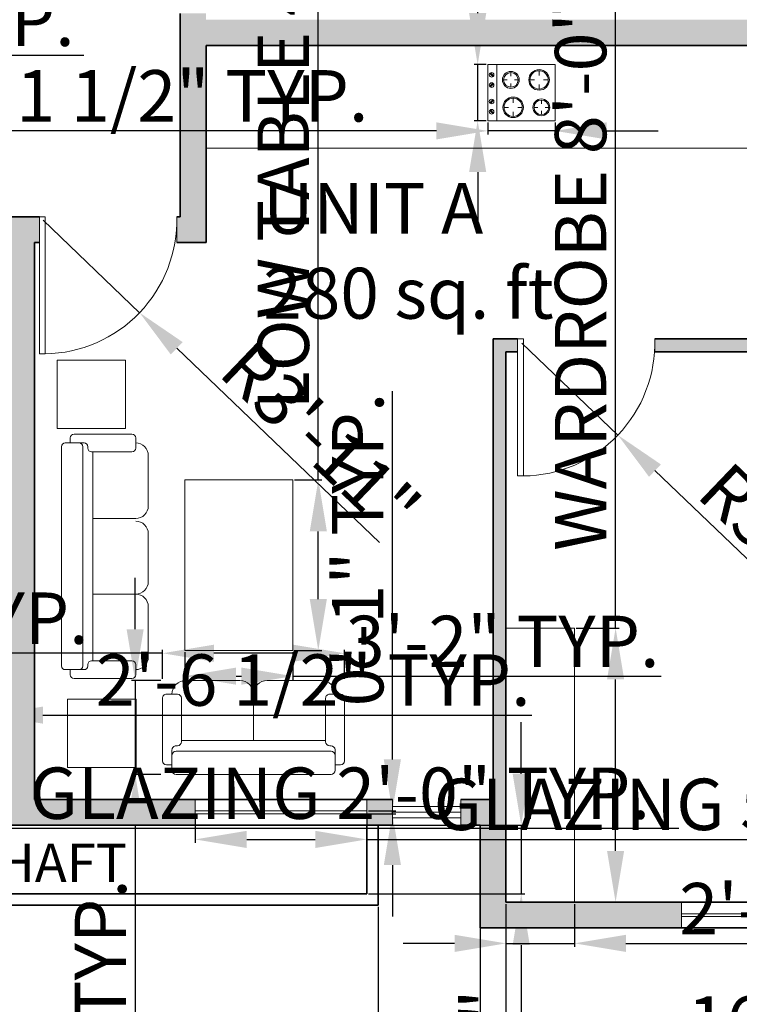
# Model space of a CAD drawing. Units: inches. Extents: x 2043 to 3177, y 1429 to 2563.
# Tile 7 of 14: x 2607 to 2858, y 1608 to 1952. Entities that reach past the tile are written whole.
import ezdxf

# ---------------------------------------------------------------- set-up
doc = ezdxf.new("R2010")
doc.units = ezdxf.units.IN
for name, color, linetype, lineweight in [('A-ANNO-DIMS', 2, 'Continuous', 13), ('A-AREA-IDEN', 7, 'Continuous', 18), ('A-DOOR', 3, 'Continuous', 18), ('A-EQPM', 8, 'Continuous', 18), ('A-FLOR-CASE', 8, 'Continuous', 18), ('A-FURN', 8, 'Continuous', 18), ('A-GLAZ', 4, 'Continuous', 18), ('A-WALL', 7, 'Continuous', 35)]:
    doc.layers.add(name, color=color, linetype=linetype, lineweight=lineweight)
doc.layers.add('A-WALL-PATT', color=251, linetype='Continuous', lineweight=13, true_color=0x636466)
doc.styles.get("Standard").update_dxf_attribs({"font": 'arial.ttf'})
doc.dimstyles.new('ISO-25', dxfattribs={"dimtxt": 18, "dimasz": 18, "dimexe": 1.25, "dimexo": 0.625, "dimtad": 1, "dimlunit": 3, "dimtxsty": 'Standard', "dimcen": 2.5, "dimadec": 0, "dimazin": 0, "dimtfac": 1, "dimtmove": 0, "dimatfit": 3, "dimfxl": 1, "dimarcsym": 0})

# ---------------------------------------------------------------- blocks, each defined once
blk = doc.blocks.new('A$C115861F8')
for p, q in [((0.0679, 0.6401), (0.0679, 0.6013)), ((1.7846, 0.6692), (0.097, 0.6692)), ((1.8136, 0.6401), (1.8136, 0.6013)), ((0, 0.5722), (0, 0.1261)), ((0.0679, 0.6013), (0.0291, 0.6013)), ((0.0679, 0.5334), (0.0679, 0.6013)), ((0.0679, 0.4946), (0.0679, 0.5431)), ((1.8136, 0.6013), (1.8524, 0.6013)), ((1.8136, 0.5334), (1.8136, 0.6013)), ((1.8136, 0.4946), (1.8136, 0.5431)), ((1.8815, 0.5722), (1.8815, 0.1261)), ((1.7846, 0.5043), (0.097, 0.5043)), ((0.1067, 0.4655), (0.097, 0.4655)), ((1.7749, 0.4655), (1.7846, 0.4655)), ((0.1358, 0.1261), (0.1358, 0.4364)), ((1.7458, 0.4267), (0.1358, 0.4267)), ((0.6498, 0.097), (0.6498, 0.4267)), ((1.2317, 0.097), (1.2317, 0.4267)), ((1.7458, 0.1261), (1.7458, 0.4364)), ((0.0291, 0.097), (0.1067, 0.097)), ((1.8524, 0.097), (1.7749, 0.097)), ((0.1649, 0), (0.5528, 0)), ((1.1347, 0), (0.7468, 0)), ((1.3287, 0), (1.7167, 0))]:
    blk.add_line(p, q)
for centre, radius, start, end in [((0.097, 0.6401), 0.0291, 90, 180), ((1.7846, 0.6401), 0.0291, 0, 90), ((0.0291, 0.5722), 0.0291, 90, 180), ((0.097, 0.5334), 0.0291, 180, 270), ((1.7846, 0.5334), 0.0291, 270, 0), ((1.8524, 0.5722), 0.0291, 0, 90), ((0.097, 0.4946), 0.0291, 180, 270), ((0.1067, 0.4364), 0.0291, 0, 90), ((1.7749, 0.4364), 0.0291, 90, 180), ((1.7846, 0.4946), 0.0291, 270, 0), ((0.0291, 0.1261), 0.0291, 180, 270), ((0.1649, 0.097), 0.097, 180, 270), ((0.1067, 0.1261), 0.0291, 270, 0), ((0.5528, 0.097), 0.097, 270, 0), ((0.7468, 0.097), 0.097, 180, 270), ((1.1147, 0.097), 0.097, 270, 0), ((1.3287, 0.097), 0.097, 180, 270), ((1.7167, 0.097), 0.097, 270, 0), ((1.7749, 0.1261), 0.0291, 180, 270), ((1.8524, 0.1261), 0.0291, 270, 0)]:
    blk.add_arc(centre, radius, start, end)
blk = doc.blocks.new('A$C02A636C4')
for p, q in [((0.0679, 0.6401), (0.0679, 0.6013)), ((1.2026, 0.6692), (0.097, 0.6692)), ((1.2317, 0.6401), (1.2317, 0.6013)), ((0, 0.5722), (0, 0.1261)), ((0.0679, 0.6013), (0.0291, 0.6013)), ((0.0679, 0.5334), (0.0679, 0.6013)), ((1.2317, 0.6013), (1.2705, 0.6013)), ((1.2317, 0.5334), (1.2317, 0.6013)), ((1.2996, 0.5722), (1.2996, 0.1261)), ((0.0679, 0.4946), (0.0679, 0.5431)), ((1.2026, 0.5043), (0.097, 0.5043)), ((1.2317, 0.4946), (1.2317, 0.5431)), ((0.1067, 0.4655), (0.097, 0.4655)), ((0.1358, 0.1261), (0.1358, 0.4364)), ((1.1638, 0.4267), (0.1358, 0.4267)), ((0.6498, 0.097), (0.6498, 0.4267)), ((1.1638, 0.1261), (1.1638, 0.4364)), ((1.1929, 0.4655), (1.2026, 0.4655)), ((0.0291, 0.097), (0.1067, 0.097)), ((1.2705, 0.097), (1.1929, 0.097)), ((0.1649, 0), (0.5528, 0)), ((0.7468, 0), (1.1347, 0))]:
    blk.add_line(p, q)
for centre, radius, start, end in [((0.097, 0.6401), 0.0291, 90, 180), ((1.2026, 0.6401), 0.0291, 0, 90), ((0.0291, 0.5722), 0.0291, 90, 180), ((1.2705, 0.5722), 0.0291, 0, 90), ((0.097, 0.5334), 0.0291, 180, 270), ((0.097, 0.4946), 0.0291, 180, 270), ((1.2026, 0.5334), 0.0291, 270, 0), ((1.2026, 0.4946), 0.0291, 270, 0), ((0.1067, 0.4364), 0.0291, 0, 90), ((1.1929, 0.4364), 0.0291, 90, 180), ((0.0291, 0.1261), 0.0291, 180, 270), ((0.1649, 0.097), 0.097, 180, 270), ((0.1067, 0.1261), 0.0291, 270, 0), ((0.5528, 0.097), 0.097, 270, 0), ((0.7468, 0.097), 0.097, 180, 270), ((1.1347, 0.097), 0.097, 270, 0), ((1.1929, 0.1261), 0.0291, 180, 270), ((1.2705, 0.1261), 0.0291, 270, 0)]:
    blk.add_arc(centre, radius, start, end)
blk = doc.blocks.new('*D20')
at = {"layer": 'A-ANNO-DIMS', "color": 0, "lineweight": -2, "transparency": 16777216}
for p, q in [((2767.74, 1633.77), (2767.74, 1562.86)), ((2980.74, 1633.77), (2980.74, 1562.86)), ((2785.74, 1564.11), (2962.74, 1564.11))]:
    blk.add_line(p, q, dxfattribs=at)
at = {"layer": 'A-ANNO-DIMS', "color": 0, "transparency": 16777216}
for points in [[(2785.74, 1567.11), (2785.74, 1561.11), (2767.74, 1564.11)], [(2962.74, 1567.11), (2962.74, 1561.11), (2980.74, 1564.11)]]:
    blk.add_solid(points, dxfattribs=at)
at = {"layer": 'Defpoints', "color": 0, "transparency": 16777216}
for p in [(2767.74, 1634.39), (2980.74, 1634.39), (2980.74, 1564.11)]:
    blk.add_point(p, dxfattribs=at)
at = {"layer": 'A-ANNO-DIMS', "color": 0, "transparency": 16777216, "insert": (2874.24, 1573.93), "char_height": 18, "attachment_point": 5}
blk.add_mtext('22\'-0"', dxfattribs=at)
blk = doc.blocks.new('*D21')
at = {"layer": 'A-ANNO-DIMS', "color": 0, "lineweight": -2, "transparency": 16777216}
for p, q in [((2731.99, 1641.77), (2731.99, 1511.06)), ((2767.74, 1641.77), (2767.74, 1511.06)), ((2713.99, 1512.31), (2695.99, 1512.31)), ((2731.99, 1512.31), (2767.74, 1512.31)), ((2785.74, 1512.31), (2852.83, 1512.31))]:
    blk.add_line(p, q, dxfattribs=at)
at = {"layer": 'A-ANNO-DIMS', "color": 0, "transparency": 16777216}
for points in [[(2713.99, 1515.31), (2713.99, 1509.31), (2731.99, 1512.31)], [(2785.74, 1515.31), (2785.74, 1509.31), (2767.74, 1512.31)]]:
    blk.add_solid(points, dxfattribs=at)
at = {"layer": 'Defpoints', "color": 0, "transparency": 16777216}
for p in [(2731.99, 1642.39), (2767.74, 1642.39), (2767.74, 1512.31)]:
    blk.add_point(p, dxfattribs=at)
at = {"layer": 'A-ANNO-DIMS', "color": 0, "transparency": 16777216, "insert": (2828.29, 1522.13), "char_height": 18, "attachment_point": 5}
blk.add_mtext('3\'-0"', dxfattribs=at)
blk = doc.blocks.new('*D22')
at = {"layer": 'A-ANNO-DIMS', "color": 0, "lineweight": -2, "transparency": 16777216}
for p, q in [((2482.49, 1641.77), (2482.49, 1560.37)), ((2731.99, 1641.77), (2731.99, 1560.37)), ((2500.49, 1561.62), (2713.99, 1561.62))]:
    blk.add_line(p, q, dxfattribs=at)
at = {"layer": 'A-ANNO-DIMS', "color": 0, "transparency": 16777216}
for points in [[(2500.49, 1564.62), (2500.49, 1558.62), (2482.49, 1561.62)], [(2713.99, 1564.62), (2713.99, 1558.62), (2731.99, 1561.62)]]:
    blk.add_solid(points, dxfattribs=at)
at = {"layer": 'Defpoints', "color": 0, "transparency": 16777216}
for p in [(2482.49, 1642.39), (2731.99, 1642.39), (2731.99, 1561.62)]:
    blk.add_point(p, dxfattribs=at)
at = {"layer": 'A-ANNO-DIMS', "color": 0, "transparency": 16777216, "insert": (2607.24, 1571.44), "char_height": 18, "attachment_point": 5}
blk.add_mtext('25\'-0"', dxfattribs=at)
blk = doc.blocks.new('*D29')
at = {"layer": 'A-ANNO-DIMS', "color": 0, "lineweight": -2, "transparency": 16777216}
for p, q in [((2233.74, 1633.77), (2233.74, 1430.58)), ((2980.74, 1633.77), (2980.74, 1430.58)), ((2251.74, 1431.83), (2962.74, 1431.83))]:
    blk.add_line(p, q, dxfattribs=at)
at = {"layer": 'A-ANNO-DIMS', "color": 0, "transparency": 16777216}
for points in [[(2251.74, 1434.83), (2251.74, 1428.83), (2233.74, 1431.83)], [(2962.74, 1434.83), (2962.74, 1428.83), (2980.74, 1431.83)]]:
    blk.add_solid(points, dxfattribs=at)
at = {"layer": 'Defpoints', "color": 0, "transparency": 16777216}
for p in [(2233.74, 1634.39), (2980.74, 1634.39), (2980.74, 1431.83)]:
    blk.add_point(p, dxfattribs=at)
at = {"layer": 'A-ANNO-DIMS', "color": 0, "transparency": 16777216, "insert": (2607.24, 1441.64), "char_height": 18, "attachment_point": 5}
blk.add_mtext('75\'-0"', dxfattribs=at)
blk = doc.blocks.new('A$C16A60262')
at = {"linetype": 'ByBlock'}
for p, q in [((0, 600), (0, 0)), ((487.7, 600), (0, 600)), ((0, 600), (500, 600)), ((0, 600), (500, 600)), ((500, 600), (500, 0)), ((500, 600), (500, 0)), ((500, 520.4), (0, 520.4)), ((119.4, 455.6), (119.4, 414.9)), ((363.3, 459.6), (363.3, 427.1)), ((38.1, 374.3), (78.8, 374.3)), ((200.7, 374.3), (160.1, 374.3)), ((298.2, 394.6), (330.7, 394.6)), ((363.3, 329.6), (363.3, 362.1)), ((428.3, 394.6), (395.8, 394.6)), ((119.4, 293), (119.4, 333.7)), ((119.4, 188.6), (119.4, 156.1)), ((363.3, 225.2), (363.3, 184.6)), ((54.4, 123.6), (86.9, 123.6)), ((119.4, 58.6), (119.4, 91.1)), ((184.4, 123.6), (151.9, 123.6)), ((282, 143.9), (322.6, 143.9)), ((363.3, 62.6), (363.3, 103.3)), ((444.5, 143.9), (403.9, 143.9)), ((0, 0), (500, 0))]:
    blk.add_line(p, q, dxfattribs=at)
for p, q in [((66.2, 557.5), (87.4, 578.7)), ((71.9, 551.8), (66.2, 557.5)), ((93.1, 573), (71.9, 551.8)), ((87.4, 578.7), (93.1, 573)), ((157.6, 572.5), (163.3, 578.1)), ((178.8, 551.2), (157.6, 572.5)), ((163.3, 578.1), (184.5, 556.9)), ((184.5, 556.9), (178.8, 551.2)), ((305.1, 572.5), (310.8, 578.1)), ((326.3, 551.2), (305.1, 572.5)), ((310.8, 578.1), (332, 556.9)), ((332, 556.9), (326.3, 551.2)), ((396.2, 558.5), (417.4, 579.7)), ((401.9, 552.8), (396.2, 558.5)), ((423.1, 574), (401.9, 552.8)), ((417.4, 579.7), (423.1, 574))]:
    blk.add_line(p, q)
for centre in [(80.1, 565.7), (171.2, 565.7), (317.6, 565.7), (408.7, 565.7)]:
    blk.add_circle(centre, 20.6)
for centre, radius in [((119.4, 374.3), 91.3), ((119.4, 374.3), 81.3), ((363.3, 394.6), 75), ((363.3, 394.6), 65), ((119.4, 123.6), 75), ((119.4, 123.6), 65), ((363.3, 143.9), 91.3), ((363.3, 143.9), 81.3)]:
    blk.add_circle(centre, radius, dxfattribs=at)
blk = doc.blocks.new('WARDROBE-96X24')
for p, q in [((0, 96), (24, 96)), ((24, 96), (24, 0))]:
    blk.add_line(p, q)
blk = doc.blocks.new('END-TABLE-24')
blk.add_lwpolyline([(24, 24), (24, 0), (0, 0), (0, 24)], close=True)
blk = doc.blocks.new('COFFEE-TABLE-RECT')
blk.add_lwpolyline([(0, 59.71), (37.81, 59.71), (37.81, 0), (0, 0)], close=True)
blk = doc.blocks.new('GLAZING-72')
for p, q in [((72, 1), (0, 1)), ((72, 0), (0, 0))]:
    blk.add_line(p, q)
blk = doc.blocks.new('GLAZING-24-TRIPLE')
for p, q in [((24, 4), (0, 4)), ((24, 2), (0, 2)), ((24, 0), (0, 0))]:
    blk.add_line(p, q)
blk = doc.blocks.new('GLAZING-60')
for p, q in [((0, 1), (60, 1)), ((0, 0), (60, 0))]:
    blk.add_line(p, q)
blk = doc.blocks.new('*D41')
at = {"layer": 'A-ANNO-DIMS', "color": 0, "lineweight": -2, "transparency": 16777216}
for p, q in [((2711.06, 1791.23), (2711.06, 2126.25)), ((2702.73, 1791.23), (2712.31, 1791.23)), ((2711.06, 1749.52), (2711.06, 1773.23)), ((2702.73, 1731.52), (2712.31, 1731.52))]:
    blk.add_line(p, q, dxfattribs=at)
at = {"layer": 'A-ANNO-DIMS', "color": 0, "transparency": 16777216}
for points in [[(2708.06, 1773.23), (2714.06, 1773.23), (2711.06, 1791.23)], [(2708.06, 1749.52), (2714.06, 1749.52), (2711.06, 1731.52)]]:
    blk.add_solid(points, dxfattribs=at)
at = {"layer": 'Defpoints', "color": 0, "transparency": 16777216}
for p in [(2702.11, 1791.23), (2711.06, 1791.23), (2702.11, 1731.52)]:
    blk.add_point(p, dxfattribs=at)
at = {"layer": 'A-ANNO-DIMS', "color": 0, "transparency": 16777216, "insert": (2701.13, 1967.74), "char_height": 18, "attachment_point": 5, "rotation": 90}
blk.add_mtext('LOW TABLE 4\'-11 1/2" TYP.', dxfattribs=at)
blk = doc.blocks.new('*D42')
at = {"layer": 'A-ANNO-DIMS', "color": 0, "lineweight": -2, "transparency": 16777216}
for p, q in [((2664.29, 1730.9), (2664.29, 1721.31)), ((2702.11, 1730.9), (2702.11, 1721.31)), ((2682.29, 1722.56), (2684.11, 1722.56)), ((2702.11, 1722.56), (2831.06, 1722.56))]:
    blk.add_line(p, q, dxfattribs=at)
at = {"layer": 'A-ANNO-DIMS', "color": 0, "transparency": 16777216}
for points in [[(2682.29, 1725.56), (2682.29, 1719.56), (2664.29, 1722.56)], [(2684.11, 1725.56), (2684.11, 1719.56), (2702.11, 1722.56)]]:
    blk.add_solid(points, dxfattribs=at)
at = {"layer": 'Defpoints', "color": 0, "transparency": 16777216}
for p in [(2664.29, 1731.52), (2702.11, 1731.52), (2702.11, 1722.56)]:
    blk.add_point(p, dxfattribs=at)
at = {"layer": 'A-ANNO-DIMS', "color": 0, "transparency": 16777216, "insert": (2775.59, 1732.38), "char_height": 18, "attachment_point": 5}
blk.add_mtext('3\'-2" TYP.', dxfattribs=at)
blk = doc.blocks.new('*D44')
at = {"layer": 'A-ANNO-DIMS', "color": 0, "lineweight": -2, "transparency": 16777216}
for p, q in [((2566.23, 1721.12), (2566.23, 1707.66)), ((2596.65, 1721.12), (2596.65, 1707.66)), ((2548.23, 1708.91), (2530.23, 1708.91)), ((2566.23, 1708.91), (2596.65, 1708.91)), ((2614.65, 1708.91), (2785.87, 1708.91))]:
    blk.add_line(p, q, dxfattribs=at)
at = {"layer": 'A-ANNO-DIMS', "color": 0, "transparency": 16777216}
for points in [[(2548.23, 1711.91), (2548.23, 1705.91), (2566.23, 1708.91)], [(2614.65, 1711.91), (2614.65, 1705.91), (2596.65, 1708.91)]]:
    blk.add_solid(points, dxfattribs=at)
at = {"layer": 'Defpoints', "color": 0, "transparency": 16777216}
for p in [(2566.23, 1721.74), (2596.65, 1721.74), (2596.65, 1708.91)]:
    blk.add_point(p, dxfattribs=at)
at = {"layer": 'A-ANNO-DIMS', "color": 0, "transparency": 16777216, "insert": (2709.26, 1718.85), "char_height": 18, "attachment_point": 5}
blk.add_mtext('2\'-6 1/2" TYP.', dxfattribs=at)
blk = doc.blocks.new('*D45')
at = {"layer": 'A-ANNO-DIMS', "color": 0, "lineweight": -2, "transparency": 16777216}
for p, q in [((2656.49, 1721.63), (2656.49, 1731.82)), ((2720.27, 1721.63), (2720.27, 1731.82)), ((2656.49, 1730.57), (2388.57, 1730.57)), ((2702.27, 1730.57), (2674.49, 1730.57))]:
    blk.add_line(p, q, dxfattribs=at)
at = {"layer": 'A-ANNO-DIMS', "color": 0, "transparency": 16777216}
for points in [[(2674.49, 1733.57), (2674.49, 1727.57), (2656.49, 1730.57)], [(2702.27, 1733.57), (2702.27, 1727.57), (2720.27, 1730.57)]]:
    blk.add_solid(points, dxfattribs=at)
at = {"layer": 'Defpoints', "color": 0, "transparency": 16777216}
for p in [(2656.49, 1730.57), (2656.49, 1721), (2720.27, 1721)]:
    blk.add_point(p, dxfattribs=at)
at = {"layer": 'A-ANNO-DIMS', "color": 0, "transparency": 16777216, "insert": (2513.53, 1740.51), "char_height": 18, "attachment_point": 5}
blk.add_mtext('LOVESEAT 5\'-4" TYP.', dxfattribs=at)
blk = doc.blocks.new('*D46')
at = {"layer": 'A-ANNO-DIMS', "color": 0, "lineweight": -2, "transparency": 16777216}
for p, q in [((2646.93, 1739), (2646.93, 1757)), ((2655.87, 1721), (2645.68, 1721)), ((2646.93, 1721), (2646.93, 1688.16)), ((2655.87, 1688.16), (2645.68, 1688.16)), ((2646.93, 1670.16), (2646.93, 1540.89))]:
    blk.add_line(p, q, dxfattribs=at)
at = {"layer": 'A-ANNO-DIMS', "color": 0, "transparency": 16777216}
for points in [[(2643.93, 1739), (2649.93, 1739), (2646.93, 1721)], [(2643.93, 1670.16), (2649.93, 1670.16), (2646.93, 1688.16)]]:
    blk.add_solid(points, dxfattribs=at)
at = {"layer": 'Defpoints', "color": 0, "transparency": 16777216}
for p in [(2656.49, 1721), (2646.93, 1688.16), (2656.49, 1688.16)]:
    blk.add_point(p, dxfattribs=at)
at = {"layer": 'A-ANNO-DIMS', "color": 0, "transparency": 16777216, "insert": (2637.11, 1596.52), "char_height": 18, "attachment_point": 5, "rotation": 90}
blk.add_mtext('2\'-9" TYP.', dxfattribs=at)
blk = doc.blocks.new('*D57')
at = {"layer": 'A-ANNO-DIMS', "color": 0, "lineweight": -2, "transparency": 16777216}
for p, q in [((2309.03, 1935.24), (2309.03, 1941.18)), ((2344.46, 1935.24), (2344.46, 1941.18)), ((2291.03, 1939.93), (2273.03, 1939.93)), ((2309.03, 1939.93), (2344.46, 1939.93)), ((2362.46, 1939.93), (2629.01, 1939.93))]:
    blk.add_line(p, q, dxfattribs=at)
at = {"layer": 'A-ANNO-DIMS', "color": 0, "transparency": 16777216}
for points in [[(2291.03, 1942.93), (2291.03, 1936.93), (2309.03, 1939.93)], [(2362.46, 1942.93), (2362.46, 1936.93), (2344.46, 1939.93)]]:
    blk.add_solid(points, dxfattribs=at)
at = {"layer": 'Defpoints', "color": 0, "transparency": 16777216}
for p in [(2344.46, 1939.93), (2309.03, 1934.62), (2344.46, 1934.62)]:
    blk.add_point(p, dxfattribs=at)
at = {"layer": 'A-ANNO-DIMS', "color": 0, "transparency": 16777216, "insert": (2504.74, 1949.86), "char_height": 18, "attachment_point": 5}
blk.add_mtext('BASIN 2\'-11 1/2" TYP.', dxfattribs=at)
blk = doc.blocks.new('*D61')
at = {"layer": 'A-ANNO-DIMS', "color": 0, "lineweight": -2, "transparency": 16777216}
for p, q in [((2752.39, 1913.46), (2434.98, 1913.46)), ((2770.39, 1916.38), (2770.39, 1912.21)), ((2794.01, 1913.46), (2770.39, 1913.46)), ((2794.01, 1916.38), (2794.01, 1912.21)), ((2812.01, 1913.46), (2830.01, 1913.46))]:
    blk.add_line(p, q, dxfattribs=at)
at = {"layer": 'A-ANNO-DIMS', "color": 0, "transparency": 16777216}
for points in [[(2752.39, 1916.46), (2752.39, 1910.46), (2770.39, 1913.46)], [(2812.01, 1916.46), (2812.01, 1910.46), (2794.01, 1913.46)]]:
    blk.add_solid(points, dxfattribs=at)
at = {"layer": 'Defpoints', "color": 0, "transparency": 16777216}
for p in [(2770.39, 1917.01), (2794.01, 1917.01), (2770.39, 1913.46)]:
    blk.add_point(p, dxfattribs=at)
at = {"layer": 'A-ANNO-DIMS', "color": 0, "transparency": 16777216, "insert": (2584.68, 1923.4), "char_height": 18, "attachment_point": 5}
blk.add_mtext('COOKTOP 1\'-11 1/2" TYP.', dxfattribs=at)
blk = doc.blocks.new('*D62')
at = {"layer": 'A-ANNO-DIMS', "color": 0, "lineweight": -2, "transparency": 16777216}
for p, q in [((2766.85, 1954.69), (2766.85, 2123.91)), ((2769.77, 1936.69), (2765.6, 1936.69)), ((2766.85, 1917.01), (2766.85, 1936.69)), ((2769.77, 1917.01), (2765.6, 1917.01)), ((2766.85, 1899.01), (2766.85, 1881.01))]:
    blk.add_line(p, q, dxfattribs=at)
at = {"layer": 'A-ANNO-DIMS', "color": 0, "transparency": 16777216}
for points in [[(2763.85, 1954.69), (2769.85, 1954.69), (2766.85, 1936.69)], [(2763.85, 1899.01), (2769.85, 1899.01), (2766.85, 1917.01)]]:
    blk.add_solid(points, dxfattribs=at)
at = {"layer": 'Defpoints', "color": 0, "transparency": 16777216}
for p in [(2766.85, 1936.69), (2770.39, 1936.69), (2770.39, 1917.01)]:
    blk.add_point(p, dxfattribs=at)
at = {"layer": 'A-ANNO-DIMS', "color": 0, "transparency": 16777216, "insert": (2756.92, 2048.3), "char_height": 18, "attachment_point": 5, "rotation": 90}
blk.add_mtext('1\'-7 1/2" TYP.', dxfattribs=at)
blk = doc.blocks.new('*D65')
at = {"layer": 'A-ANNO-DIMS', "color": 0, "lineweight": -2, "transparency": 16777216}
for p, q in [((2815.14, 1739.39), (2815.14, 2024.17)), ((2801.37, 1739.39), (2816.39, 1739.39)), ((2815.14, 1661.39), (2815.14, 1721.39)), ((2801.37, 1643.39), (2816.39, 1643.39))]:
    blk.add_line(p, q, dxfattribs=at)
at = {"layer": 'A-ANNO-DIMS', "color": 0, "transparency": 16777216}
for points in [[(2812.14, 1721.39), (2818.14, 1721.39), (2815.14, 1739.39)], [(2812.14, 1661.39), (2818.14, 1661.39), (2815.14, 1643.39)]]:
    blk.add_solid(points, dxfattribs=at)
at = {"layer": 'Defpoints', "color": 0, "transparency": 16777216}
for p in [(2800.74, 1739.39), (2815.14, 1739.39), (2800.74, 1643.39)]:
    blk.add_point(p, dxfattribs=at)
at = {"layer": 'A-ANNO-DIMS', "color": 0, "transparency": 16777216, "insert": (2805.21, 1890.78), "char_height": 18, "attachment_point": 5, "rotation": 90}
blk.add_mtext('WARDROBE 8\'-0" TYP.', dxfattribs=at)
blk = doc.blocks.new('*D66')
at = {"layer": 'A-ANNO-DIMS', "color": 0, "lineweight": -2, "transparency": 16777216}
for p, q in [((2776.74, 1642.77), (2776.74, 1627.74)), ((2800.74, 1642.77), (2800.74, 1627.74)), ((2758.74, 1628.99), (2740.74, 1628.99)), ((2776.74, 1628.99), (2800.74, 1628.99)), ((2818.74, 1628.99), (2948.02, 1628.99))]:
    blk.add_line(p, q, dxfattribs=at)
at = {"layer": 'A-ANNO-DIMS', "color": 0, "transparency": 16777216}
for points in [[(2758.74, 1631.99), (2758.74, 1625.99), (2776.74, 1628.99)], [(2818.74, 1631.99), (2818.74, 1625.99), (2800.74, 1628.99)]]:
    blk.add_solid(points, dxfattribs=at)
at = {"layer": 'Defpoints', "color": 0, "transparency": 16777216}
for p in [(2776.74, 1643.39), (2800.74, 1643.39), (2800.74, 1628.99)]:
    blk.add_point(p, dxfattribs=at)
at = {"layer": 'A-ANNO-DIMS', "color": 0, "transparency": 16777216, "insert": (2892.38, 1638.81), "char_height": 18, "attachment_point": 5}
blk.add_mtext('2\'-0" TYP.', dxfattribs=at)
blk = doc.blocks.new('*D67')
at = {"layer": 'A-ANNO-DIMS', "color": 0, "lineweight": -2, "transparency": 16777216}
for p, q in [((2453.49, 1672.27), (2453.49, 1668.04)), ((2477.49, 1672.27), (2477.49, 1668.04)), ((2435.49, 1669.29), (2417.49, 1669.29)), ((2453.49, 1669.29), (2477.49, 1669.29)), ((2495.49, 1669.29), (2837.31, 1669.29))]:
    blk.add_line(p, q, dxfattribs=at)
at = {"layer": 'A-ANNO-DIMS', "color": 0, "transparency": 16777216}
for points in [[(2435.49, 1672.29), (2435.49, 1666.29), (2453.49, 1669.29)], [(2495.49, 1672.29), (2495.49, 1666.29), (2477.49, 1669.29)]]:
    blk.add_solid(points, dxfattribs=at)
at = {"layer": 'Defpoints', "color": 0, "transparency": 16777216}
for p in [(2453.49, 1672.89), (2477.49, 1672.89), (2477.49, 1669.29)]:
    blk.add_point(p, dxfattribs=at)
at = {"layer": 'A-ANNO-DIMS', "color": 0, "transparency": 16777216, "insert": (2675.4, 1679.23), "char_height": 18, "attachment_point": 5}
blk.add_mtext('TRIPLE GLAZING 2\'-0" TYP.', dxfattribs=at)
blk = doc.blocks.new('*D69')
at = {"layer": 'A-ANNO-DIMS', "color": 0, "lineweight": -2, "transparency": 16777216}
for p, q in [((2667.99, 1673.77), (2667.99, 1664.14)), ((2727.99, 1673.77), (2727.99, 1664.14)), ((2685.99, 1665.39), (2709.99, 1665.39)), ((2727.99, 1665.39), (2974.04, 1665.39))]:
    blk.add_line(p, q, dxfattribs=at)
at = {"layer": 'A-ANNO-DIMS', "color": 0, "transparency": 16777216}
for points in [[(2685.99, 1668.39), (2685.99, 1662.39), (2667.99, 1665.39)], [(2709.99, 1668.39), (2709.99, 1662.39), (2727.99, 1665.39)]]:
    blk.add_solid(points, dxfattribs=at)
at = {"layer": 'Defpoints', "color": 0, "transparency": 16777216}
for p in [(2667.99, 1674.39), (2727.99, 1674.39), (2727.99, 1665.39)]:
    blk.add_point(p, dxfattribs=at)
at = {"layer": 'A-ANNO-DIMS', "color": 0, "transparency": 16777216, "insert": (2860.02, 1675.33), "char_height": 18, "attachment_point": 5}
blk.add_mtext('GLAZING 5\'-0" TYP.', dxfattribs=at)
blk = doc.blocks.new('*D70')
at = {"layer": 'A-ANNO-DIMS', "color": 0, "lineweight": -2, "transparency": 16777216}
for p, q in [((2736.99, 1693.39), (2736.99, 1822.36)), ((2728.62, 1675.39), (2738.24, 1675.39)), ((2728.62, 1674.39), (2738.24, 1674.39)), ((2736.99, 1674.39), (2736.99, 1675.39)), ((2736.99, 1656.39), (2736.99, 1638.39))]:
    blk.add_line(p, q, dxfattribs=at)
at = {"layer": 'A-ANNO-DIMS', "color": 0, "transparency": 16777216}
for points in [[(2733.99, 1693.39), (2739.99, 1693.39), (2736.99, 1675.39)], [(2733.99, 1656.39), (2739.99, 1656.39), (2736.99, 1674.39)]]:
    blk.add_solid(points, dxfattribs=at)
at = {"layer": 'Defpoints', "color": 0, "transparency": 16777216}
for p in [(2727.99, 1675.39), (2727.99, 1674.39), (2736.99, 1675.39)]:
    blk.add_point(p, dxfattribs=at)
at = {"layer": 'A-ANNO-DIMS', "color": 0, "transparency": 16777216, "insert": (2727.18, 1766.88), "char_height": 18, "attachment_point": 5, "rotation": 90}
blk.add_mtext('0\'-1" TYP.', dxfattribs=at)
blk = doc.blocks.new('*D75')
at = {"layer": 'A-ANNO-DIMS', "color": 0, "lineweight": -2, "transparency": 16777216}
for p, q in [((2776.74, 1642.77), (2776.74, 1588.04)), ((2971.74, 1642.77), (2971.74, 1588.04)), ((2953.74, 1589.29), (2794.74, 1589.29))]:
    blk.add_line(p, q, dxfattribs=at)
at = {"layer": 'A-ANNO-DIMS', "color": 0, "transparency": 16777216}
for points in [[(2794.74, 1592.29), (2794.74, 1586.29), (2776.74, 1589.29)], [(2953.74, 1592.29), (2953.74, 1586.29), (2971.74, 1589.29)]]:
    blk.add_solid(points, dxfattribs=at)
at = {"layer": 'Defpoints', "color": 0, "transparency": 16777216}
for p in [(2776.74, 1643.39), (2971.74, 1643.39), (2776.74, 1589.29)]:
    blk.add_point(p, dxfattribs=at)
at = {"layer": 'A-ANNO-DIMS', "color": 0, "transparency": 16777216, "insert": (2874.24, 1599.11), "char_height": 18, "attachment_point": 5}
blk.add_mtext('16\'-3"', dxfattribs=at)
blk = doc.blocks.new('*D81')
at = {"layer": 'A-ANNO-DIMS', "color": 0, "lineweight": -2, "transparency": 16777216}
for p, q in [((2782.09, 1688.39), (2782.09, 1706.39)), ((2728.62, 1670.39), (2783.34, 1670.39)), ((2782.09, 1670.39), (2782.09, 1646.39)), ((2728.62, 1646.39), (2783.34, 1646.39)), ((2782.09, 1628.39), (2782.09, 1560.99))]:
    blk.add_line(p, q, dxfattribs=at)
at = {"layer": 'A-ANNO-DIMS', "color": 0, "transparency": 16777216}
for points in [[(2779.09, 1688.39), (2785.09, 1688.39), (2782.09, 1670.39)], [(2779.09, 1628.39), (2785.09, 1628.39), (2782.09, 1646.39)]]:
    blk.add_solid(points, dxfattribs=at)
at = {"layer": 'Defpoints', "color": 0, "transparency": 16777216}
for p in [(2727.99, 1670.39), (2727.99, 1646.39), (2782.09, 1646.39)]:
    blk.add_point(p, dxfattribs=at)
at = {"layer": 'A-ANNO-DIMS', "color": 0, "transparency": 16777216, "insert": (2772.28, 1585.69), "char_height": 18, "attachment_point": 5, "rotation": 90}
blk.add_mtext('2\'-0"', dxfattribs=at)
blk = doc.blocks.new('*D84')
at = {"layer": 'A-ANNO-DIMS', "color": 0, "lineweight": -2, "transparency": 16777216}
for p, q in [((2614.69, 1882.19), (2648.48, 1849.81)), ((2732.45, 1769.33), (2661.47, 1837.35))]:
    blk.add_line(p, q, dxfattribs=at)
at = {"layer": 'A-ANNO-DIMS', "color": 0, "transparency": 16777216}
blk.add_solid([(2663.55, 1839.52), (2659.4, 1835.18), (2648.48, 1849.81)], dxfattribs=at)
at = {"layer": 'Defpoints', "color": 0, "transparency": 16777216}
for p in [(2614.69, 1882.19), (2648.48, 1849.81)]:
    blk.add_point(p, dxfattribs=at)
at = {"layer": 'A-ANNO-DIMS', "color": 0, "transparency": 16777216, "insert": (2710.26, 1804.2), "char_height": 18, "attachment_point": 5, "rotation": 316.2189}
blk.add_mtext('R3\'-11"', dxfattribs=at)
blk = doc.blocks.new('*D88')
at = {"layer": 'A-ANNO-DIMS', "color": 0, "lineweight": -2, "transparency": 16777216}
for p, q in [((2782.34, 1839.16), (2815.93, 1806.97)), ((2930.19, 1697.48), (2828.93, 1794.52))]:
    blk.add_line(p, q, dxfattribs=at)
at = {"layer": 'A-ANNO-DIMS', "color": 0, "transparency": 16777216}
blk.add_solid([(2831, 1796.69), (2826.85, 1792.35), (2815.93, 1806.97)], dxfattribs=at)
at = {"layer": 'Defpoints', "color": 0, "transparency": 16777216}
for p in [(2782.34, 1839.16), (2815.93, 1806.97)]:
    blk.add_point(p, dxfattribs=at)
at = {"layer": 'A-ANNO-DIMS', "color": 0, "transparency": 16777216, "insert": (2892.93, 1746.95), "char_height": 18, "attachment_point": 5, "rotation": 316.2186}
blk.add_mtext('R3\'-10 1/2"', dxfattribs=at)

msp = doc.modelspace()

# ---------------------------------------------------------------- hatches: boundary and pattern name
at = {"layer": 'A-WALL-PATT'}
h = msp.add_hatch(color=256, dxfattribs=at)
h.dxf.hatch_style = 1
h.paths.add_polyline_path([(2283.62, 2261.393), (2233.745, 2261.393), (2233.745, 2029.268), (2242.745, 2029.268), (2242.745, 2070.143), (2348.495, 2070.143), (2348.495, 2063.887), (2352.995, 2063.887), (2352.995, 2094.143), (2353.364, 2094.143, -0.017175), (2353.364, 2096.932), (2353.364, 2098.643), (2348.495, 2098.643), (2348.495, 2096.393), (2348.495, 2074.643), (2242.745, 2074.643), (2242.745, 2252.393), (2283.62, 2252.393)])
h.paths.add_polyline_path([(2453.87, 2261.393), (2355.62, 2261.393), (2355.62, 2252.393), (2396.495, 2252.393), (2396.495, 2098.643), (2395.364, 2098.643), (2395.364, 2094.143), (2436.995, 2094.143), (2436.995, 2098.643), (2400.995, 2098.643), (2400.995, 2252.393), (2453.87, 2252.393)])
h.paths.add_polyline_path([(2551.745, 2261.393), (2489.87, 2261.393), (2489.87, 2252.393), (2542.745, 2252.393), (2542.745, 2098.643), (2506.745, 2098.643), (2506.745, 2094.143), (2542.745, 2094.143), (2542.745, 2003.513), (2549.809, 2003.513, -0.0102854), (2551.745, 2003.513), (2551.745, 2195.393), (2571.245, 2195.393), (2571.245, 2204.393), (2551.745, 2204.393)])
h.paths.add_polyline_path([(2724.62, 2261.393), (2662.745, 2261.393), (2662.745, 2204.393), (2643.245, 2204.393), (2643.245, 2195.393), (2662.745, 2195.393), (2662.745, 2002.566, -0.0156152), (2665.651, 2002.566), (2671.745, 2002.566), (2671.745, 2094.143), (2707.745, 2094.143), (2707.745, 2098.643), (2671.745, 2098.643), (2671.745, 2252.393), (2724.62, 2252.393)])
h.paths.add_polyline_path([(2858.87, 2261.393), (2760.62, 2261.393), (2760.62, 2252.393), (2813.495, 2252.393), (2813.495, 2098.643), (2777.495, 2098.643), (2777.495, 2094.143), (2819.302, 2094.143), (2819.302, 2098.643), (2817.995, 2098.643), (2817.995, 2252.393), (2858.87, 2252.393)])
h.paths.add_polyline_path([(2980.745, 2261.393), (2930.87, 2261.393), (2930.87, 2252.393), (2971.745, 2252.393), (2971.745, 2074.643), (2865.995, 2074.643), (2865.995, 2098.643), (2861.429, 2098.643, -0.0279128), (2861.495, 2094.143), (2861.495, 2063.254), (2865.995, 2063.254), (2865.995, 2070.143), (2971.745, 2070.143), (2971.745, 2029.268), (2980.745, 2029.268)])
h.paths.add_polyline_path([(2980.745, 1993.268), (2971.745, 1993.268), (2971.745, 1952.393), (2865.995, 1952.393), (2865.995, 2027.254), (2865.688, 2027.254, -0.0309542), (2861.495, 2027.254), (2861.495, 1952.393), (2671.745, 1952.393), (2671.745, 1954.566), (2662.745, 1954.566), (2662.745, 1883.393), (2661.473, 1883.393, -0.012912), (2661.473, 1880.977), (2661.473, 1874.393), (2671.745, 1874.393), (2671.745, 1943.393), (2861.495, 1943.393), (2861.495, 1903.412, -0.0351753), (2865.995, 1903.659), (2865.995, 1943.393), (2971.745, 1943.393), (2971.745, 1922.018), (2980.745, 1922.018)])
h.paths.add_polyline_path([(2980.745, 1886.018), (2971.745, 1886.018), (2971.745, 1864.643), (2865.995, 1864.643), (2865.995, 1867.412), (2861.495, 1867.412), (2861.495, 1840.643), (2828.844, 1840.643, -0.0159075), (2828.844, 1837.684), (2828.844, 1836.143), (2865.995, 1836.143), (2865.995, 1860.143), (2971.745, 1860.143), (2971.745, 1643.393), (2910.245, 1643.393), (2910.245, 1634.393), (2980.745, 1634.393)])
h.paths.add_polyline_path([(2776.745, 1836.143), (2780.844, 1836.143), (2780.844, 1840.643), (2772.245, 1840.643), (2772.245, 1679.393), (2760.995, 1679.393), (2760.995, 1670.393), (2767.745, 1670.393), (2767.745, 1634.393), (2838.245, 1634.393), (2838.245, 1643.393), (2776.745, 1643.393)])
h.paths.add_polyline_path([(2736.995, 1679.393), (2727.995, 1679.393), (2727.995, 1670.393), (2736.995, 1670.393)])
h.paths.add_polyline_path([(2667.995, 1679.393), (2611.745, 1679.393), (2611.745, 1874.393), (2613.473, 1874.393), (2613.473, 1883.393), (2600.336, 1883.393), (2600.336, 1874.393), (2602.745, 1874.393), (2602.745, 1679.393), (2546.495, 1679.393), (2546.495, 1670.393), (2667.995, 1670.393)])
h.paths.add_polyline_path([(2486.495, 1679.393), (2477.495, 1679.393), (2477.495, 1670.393), (2486.495, 1670.393)])
h.paths.add_polyline_path([(2453.495, 1679.393), (2442.245, 1679.393), (2442.245, 1839.893), (2427.654, 1839.893), (2427.654, 1835.393), (2437.745, 1835.393), (2437.745, 1643.393), (2376.245, 1643.393), (2376.245, 1634.393), (2446.745, 1634.393), (2446.745, 1670.393), (2453.495, 1670.393)])
h.paths.add_polyline_path([(2304.245, 1643.393), (2242.745, 1643.393), (2242.745, 1857.143), (2348.495, 1857.143), (2348.495, 1835.393), (2352.995, 1835.393), (2379.654, 1835.393), (2379.654, 1837.073, -0.0151369), (2379.654, 1839.893), (2352.995, 1839.893), (2352.995, 1867.394), (2348.495, 1867.394), (2348.495, 1861.643), (2242.745, 1861.643), (2242.745, 1884.518), (2233.745, 1884.518), (2233.745, 1634.393), (2304.245, 1634.393)])
h.paths.add_polyline_path([(2551.745, 1955.513), (2542.745, 1955.513), (2542.745, 1952.393), (2352.995, 1952.393), (2352.995, 2027.887, -0.0208198), (2350.117, 2027.887), (2348.495, 2027.887), (2348.495, 1952.393), (2242.745, 1952.393), (2242.745, 1993.268), (2233.745, 1993.268), (2233.745, 1943.393), (2233.745, 1920.518), (2242.745, 1920.518), (2242.745, 1943.393), (2348.495, 1943.393), (2348.495, 1903.394), (2352.995, 1903.394), (2352.995, 1943.393), (2542.745, 1943.393), (2542.745, 1874.393), (2552.336, 1874.393), (2552.336, 1880.494, -0.0155728), (2552.336, 1883.393), (2551.745, 1883.393)])

# ---------------------------------------------------------------- linework, layer by layer
at = {"layer": 'A-DOOR'}
for p, q in [((2613.473, 1874.393), (2613.473, 1883.393)), ((2613.473, 1883.393), (2613.473, 1835.393)), ((2613.473, 1883.393), (2615.473, 1883.393)), ((2615.473, 1883.393), (2615.473, 1835.393)), ((2661.473, 1874.393), (2661.473, 1883.393)), ((2780.844, 1840.643), (2780.844, 1836.143)), ((2780.844, 1840.643), (2780.844, 1792.643)), ((2780.844, 1840.643), (2782.844, 1840.643)), ((2782.844, 1840.643), (2782.844, 1792.643)), ((2828.844, 1840.643), (2828.844, 1836.143)), ((2613.473, 1835.393), (2615.473, 1835.393)), ((2780.844, 1792.643), (2782.844, 1792.643))]:
    msp.add_line(p, q, dxfattribs=at)
for centre, radius, start, end in [((2614.69, 1882.185), 46.798, 270.95823, 1.47953), ((2782.344, 1839.164), 46.523, 270.61504, 1.82271)]:
    msp.add_arc(centre, radius, start, end, dxfattribs=at)
at = {"layer": 'A-FLOR-CASE'}
msp.add_line((2671.745, 1907.393), (2861.495, 1907.393), dxfattribs=at)
at = {"layer": 'A-GLAZ'}
for p, q in [((2667.995, 1679.393), (2667.995, 1670.393)), ((2727.995, 1679.393), (2727.995, 1670.393)), ((2736.995, 1679.393), (2736.995, 1670.393)), ((2760.995, 1679.393), (2760.995, 1670.393)), ((2838.245, 1643.393), (2838.245, 1634.393))]:
    msp.add_line(p, q, dxfattribs=at)
at = {"layer": 'A-WALL'}
for p, q in [((2662.745, 1883.393), (2662.745, 1954.566)), ((2671.745, 1943.393), (2861.495, 1943.393)), ((2671.745, 1874.393), (2671.745, 1943.393)), ((2600.336, 1883.393), (2613.473, 1883.393)), ((2661.473, 1883.393), (2662.745, 1883.393)), ((2611.745, 1679.393), (2611.745, 1874.393)), ((2611.745, 1874.393), (2613.473, 1874.393)), ((2661.473, 1874.393), (2671.745, 1874.393)), ((2772.245, 1840.643), (2772.245, 1679.393)), ((2772.245, 1840.643), (2780.844, 1840.643)), ((2828.844, 1840.643), (2861.495, 1840.643)), ((2776.745, 1836.143), (2776.745, 1643.393)), ((2776.745, 1836.143), (2780.844, 1836.143)), ((2828.844, 1836.143), (2865.995, 1836.143)), ((2611.745, 1679.393), (2736.995, 1679.393)), ((2760.995, 1679.393), (2772.245, 1679.393)), ((2477.495, 1670.393), (2736.995, 1670.393)), ((2727.995, 1646.393), (2727.995, 1670.393)), ((2731.995, 1642.393), (2731.995, 1670.393)), ((2760.995, 1670.393), (2767.745, 1670.393)), ((2767.745, 1634.393), (2767.745, 1670.393)), ((2486.495, 1646.393), (2727.995, 1646.393)), ((2482.495, 1642.393), (2731.995, 1642.393)), ((2776.745, 1643.393), (2971.745, 1643.393)), ((2767.745, 1634.393), (2980.745, 1634.393))]:
    msp.add_line(p, q, dxfattribs=at)

# ---------------------------------------------------------------- block references
at = {"layer": 'A-EQPM', "xscale": 0.0393700787401575, "yscale": 0.0393700787401575, "zscale": 0.0393700787401575, "rotation": 90}
msp.add_blockref('A$C16A60262', (2794.015, 1917.007), dxfattribs=at)
at = {"layer": 'A-FLOR-CASE'}
msp.add_blockref('WARDROBE-96X24', (2776.745, 1643.393), dxfattribs=at)
at = {"layer": 'A-FURN'}
for name, p in [('END-TABLE-24', (2619.571, 1809.22)), ('COFFEE-TABLE-RECT', (2664.293, 1731.521)), ('END-TABLE-24', (2623.27, 1690.549))]:
    msp.add_blockref(name, p, dxfattribs=at)
for name, p, xscale, yscale, zscale, rotation in [('A$C115861F8', (2651.542, 1721.745), 45.45990975277036, 45.45990975277036, 45.45990975277036, 90), ('A$C02A636C4', (2720.274, 1721.004), 49.07597789630211, 49.07597789630211, 49.07597789630211, 180)]:
    msp.add_blockref(name, p, dxfattribs=dict(at, xscale=xscale, yscale=yscale, zscale=zscale, rotation=rotation))
at = {"layer": 'A-GLAZ'}
for name, p in [('GLAZING-24-TRIPLE', (2736.995, 1672.893)), ('GLAZING-60', (2667.995, 1674.393)), ('GLAZING-72', (2838.245, 1638.393))]:
    msp.add_blockref(name, p, dxfattribs=at)

# ---------------------------------------------------------------- texts
at = {"layer": 'A-AREA-IDEN', "attachment_point": 1}
for s, width, gutter_width, insert, char_height in [('UNIT A \\P280 sq. ft', 505.18079, 89.135, (2691.771, 1895.254), 17.8269), ('SHAFT', 381.44992, 67.303, (2587.501, 1663.948), 13.4607)]:
    msp.add_mtext_dynamic_manual_height_columns(s, width=width, gutter_width=gutter_width, heights=[0], dxfattribs=dict(at, insert=insert, char_height=char_height))

# ---------------------------------------------------------------- dimensions: what is measured, and where the dimension line sits
at = {"layer": 'A-ANNO-DIMS'}
for base, p1, p2, angle, text, picture, middle in [((2711.065, 1791.234), (2702.108, 1731.521), (2702.108, 1791.234), 90, 'LOW TABLE <> TYP.', '*D41', (2701.127, 1967.74)), ((2766.849, 1936.692), (2770.393, 1917.007), (2770.393, 1936.692), 90, '<> TYP.', '*D62', (2756.918, 2048.301)), ((2815.145, 1739.393), (2800.745, 1643.393), (2800.745, 1739.393), 90, 'WARDROBE <> TYP.', '*D65', (2805.206, 1890.784)), ((2770.393, 1913.464), (2794.015, 1917.007), (2770.393, 1917.007), 180, 'COOKTOP <> TYP.', '*D61', (2584.685, 1923.402)), ((2736.995, 1675.393), (2727.995, 1674.393), (2727.995, 1675.393), 90, '<> TYP.', '*D70', (2727.179, 1766.878)), ((2656.494, 1730.571), (2720.274, 1721.004), (2656.494, 1721.004), 180, 'LOVESEAT <> TYP.', '*D45', (2513.532, 1740.509)), ((2646.927, 1688.162), (2656.494, 1721.004), (2656.494, 1688.162), 270, '<> TYP.', '*D46', (2637.111, 1596.524))]:
    dim = msp.add_linear_dim(base=base, p1=p1, p2=p2, angle=angle, text=text, dimstyle='ISO-25', override={"dimdec": 1, "dimlfac": 1, "dimrnd": 0, "dimzin": 1, "dimdsep": 46, "dimlunit": 4, "dimfrac": 2}, dxfattribs=at)
    dim.commit()
    dim.dimension.update_dxf_attribs({"geometry": picture, "text_midpoint": middle})
for base, p1, p2, text, override, picture, middle in [((2344.462, 1939.932), (2309.031, 1934.617), (2344.462, 1934.617), 'BASIN <> TYP.', {"dimdec": 1, "dimlfac": 1, "dimrnd": 0, "dimzin": 1, "dimdsep": 46, "dimlunit": 4, "dimfrac": 2}, '*D57', (2504.735, 1949.864)), ((2596.652, 1708.915), (2566.23, 1721.745), (2596.652, 1721.745), '<> TYP.', {"dimdec": 1, "dimlfac": 1, "dimrnd": 0, "dimzin": 1, "dimdsep": 46, "dimlunit": 4, "dimfrac": 2}, '*D44', (2709.261, 1718.847)), ((2702.108, 1722.564), (2664.293, 1731.521), (2702.108, 1731.521), '<> TYP.', {"dimdec": 1, "dimlfac": 1, "dimrnd": 0, "dimzin": 1, "dimdsep": 46, "dimlunit": 4, "dimfrac": 2}, '*D42', (2775.586, 1732.385)), ((2477.495, 1669.293), (2453.495, 1672.893), (2477.495, 1672.893), 'TRIPLE GLAZING <> TYP.', {"dimdec": 1, "dimlfac": 1, "dimrnd": 0, "dimzin": 1, "dimdsep": 46, "dimlunit": 4, "dimfrac": 2}, '*D67', (2675.401, 1679.225)), ((2727.995, 1665.393), (2667.995, 1674.393), (2727.995, 1674.393), 'GLAZING <> TYP.', {"dimdec": 1, "dimlfac": 1, "dimrnd": 0, "dimzin": 1, "dimdsep": 46, "dimlunit": 4, "dimfrac": 2}, '*D69', (2860.016, 1675.325)), ((2800.745, 1628.993), (2776.745, 1643.393), (2800.745, 1643.393), '<> TYP.', {"dimdec": 1, "dimlfac": 1, "dimrnd": 0, "dimzin": 1, "dimdsep": 46, "dimlunit": 4, "dimfrac": 2}, '*D66', (2892.383, 1638.809)), ((2731.995, 1561.62), (2482.495, 1642.393), (2731.995, 1642.393), '25\'-0"', {"dimclrd": 0, "dimclre": 0, "dimclrt": 0}, '*D22', (2607.245, 1571.436)), ((2767.745, 1512.311), (2731.995, 1642.393), (2767.745, 1642.393), '3\'-0"', {"dimclrd": 0, "dimclre": 0, "dimclrt": 0}, '*D21', (2828.288, 1522.132)), ((2980.745, 1431.826), (2233.745, 1634.393), (2980.745, 1634.393), '75\'-0"', {"dimclrd": 0, "dimclre": 0, "dimclrt": 0}, '*D29', (2607.245, 1441.642)), ((2980.745, 1564.114), (2767.745, 1634.393), (2980.745, 1634.393), '22\'-0"', {"dimclrd": 0, "dimclre": 0, "dimclrt": 0}, '*D20', (2874.245, 1573.929))]:
    dim = msp.add_linear_dim(base=base, p1=p1, p2=p2, text=text, dimstyle='ISO-25', override=override, dxfattribs=at)
    dim.commit()
    dim.dimension.update_dxf_attribs({"geometry": picture, "text_midpoint": middle})
for center, mpoint, picture, middle in [((2614.69, 1882.185), (2648.478, 1849.805), '*D84', (2710.256, 1804.204)), ((2782.344, 1839.164), (2815.933, 1806.974), '*D88', (2892.933, 1746.947))]:
    dim = msp.add_radius_dim(center=center, mpoint=mpoint, dimstyle='ISO-25', override={"dimdec": 1, "dimlfac": 1, "dimrnd": 0, "dimzin": 1, "dimdsep": 46, "dimlunit": 4, "dimfrac": 2}, dxfattribs=at)
    dim.commit()
    dim.dimension.update_dxf_attribs({"geometry": picture, "text_midpoint": middle})
for base, p1, p2, angle, picture, middle in [((2782.095, 1646.393), (2727.995, 1670.393), (2727.995, 1646.393), 270, '*D81', (2772.279, 1585.691)), ((2776.745, 1589.293), (2971.745, 1643.393), (2776.745, 1643.393), 180, '*D75', (2874.245, 1599.115))]:
    dim = msp.add_linear_dim(base=base, p1=p1, p2=p2, angle=angle, dimstyle='ISO-25', override={"dimdec": 1, "dimlfac": 1, "dimrnd": 0, "dimzin": 1, "dimdsep": 46, "dimlunit": 4, "dimfrac": 2}, dxfattribs=at)
    dim.commit()
    dim.dimension.update_dxf_attribs({"geometry": picture, "text_midpoint": middle})

doc.saveas('drawing.dxf')
